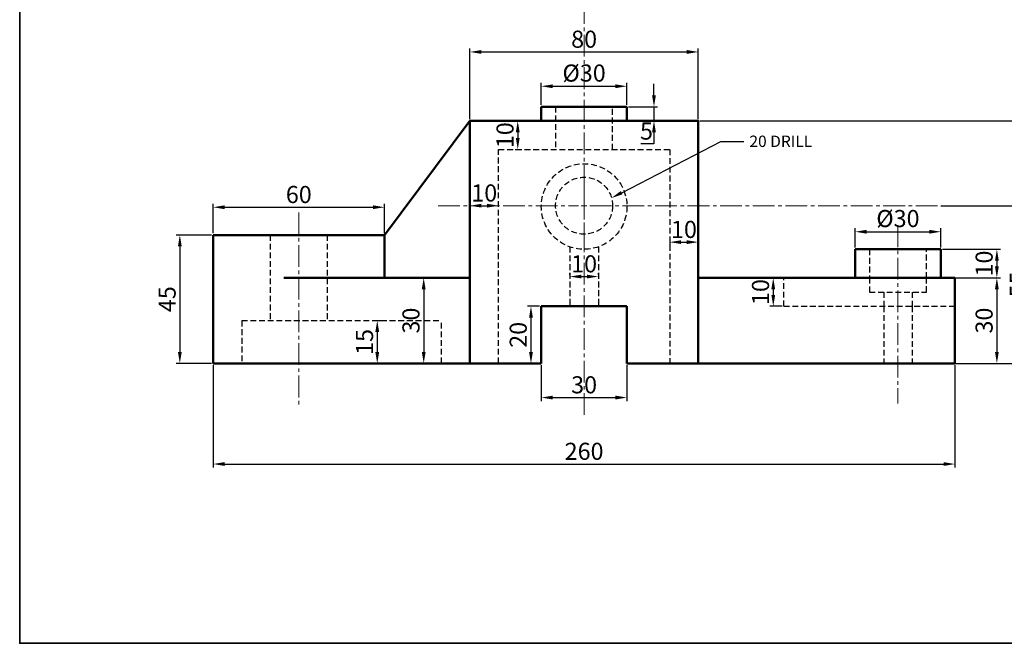
# Model space of a CAD drawing. Units: millimetres. Extents: x 33 to 569, y -180 to 232.
# Tile 1 of 3: x 33 to 378, y -180 to 39. Entities that reach past the tile are written whole.
import ezdxf
from ezdxf import colors
from ezdxf.entities.mleader import LeaderData, LeaderLine
from ezdxf.math import Vec2, Vec3

# ---------------------------------------------------------------- set-up
doc = ezdxf.new("R2010")
doc.units = ezdxf.units.MM
doc.header["$LTSCALE"] = 0.4
doc.linetypes.add('CENTER2', pattern=[28.575, 19.05, -3.175, 3.175, -3.175])
doc.linetypes.add('DASHED', pattern=[19.05, 12.7, -6.35])
for name, color, linetype, lineweight in [('M-CNTR', 1, 'CENTER2', 18), ('M-DIMS', 2, 'Continuous', 25), ('M-HIDN', 4, 'DASHED', 25), ('M-OUTL', 7, 'Continuous', 50), ('M-TEXT', 3, 'Continuous', 25), ('M-TTLB', 7, 'Continuous', 35)]:
    doc.layers.add(name, color=color, linetype=linetype, lineweight=lineweight)
doc.styles.get("Standard").update_dxf_attribs({"font": 'arial.ttf'})
doc.dimstyles.new('ISO-25', dxfattribs={"dimtxt": 6, "dimasz": 4, "dimexe": 1.25, "dimexo": 0.625, "dimtad": 1, "dimtoh": 1, "dimdec": 0, "dimtxsty": 'Standard', "dimcen": 2.5, "dimadec": 0, "dimazin": 0, "dimtfac": 1, "dimtdec": 0, "dimtmove": 0, "dimatfit": 3, "dimfxl": 1, "dimarcsym": 0})

# ---------------------------------------------------------------- blocks, each defined once
blk = doc.blocks.new('*U2')
at = {"layer": 'M-CNTR', "color": 0, "transparency": 16777216}
for p, q in [((0, 2), (0, 92.17)), ((-13.5, 0), (-2, 0)), ((2, 0), (13.5, 0)), ((0, -219.39), (0, -2))]:
    blk.add_line(p, q, dxfattribs=at)
at = {"layer": 'M-CNTR', "color": 0, "linetype": 'Continuous', "transparency": 16777216}
for p, q in [((-1, 0), (1, 0)), ((0, -1), (0, 1))]:
    blk.add_line(p, q, dxfattribs=at)
blk = doc.blocks.new('*U24')
at = {"layer": 'M-CNTR', "color": 0, "transparency": 16777216}
for p, q in [((0, 2), (0, 13.5)), ((-51.2, 0), (-2, 0)), ((2, 0), (124.4, 0)), ((0, -13.5), (0, -2))]:
    blk.add_line(p, q, dxfattribs=at)
at = {"layer": 'M-CNTR', "color": 0, "linetype": 'Continuous', "transparency": 16777216}
for p, q in [((-1, 0), (1, 0)), ((0, -1), (0, 1))]:
    blk.add_line(p, q, dxfattribs=at)
blk = doc.blocks.new('*U25')
at = {"layer": 'M-CNTR', "color": 0, "transparency": 16777216}
blk.add_line((0, 13.4), (0, -49.13), dxfattribs=at)
blk = doc.blocks.new('*U26')
at = {"layer": 'M-CNTR', "color": 0, "transparency": 16777216}
blk.add_line((0, 22.85), (0, -45.4), dxfattribs=at)
blk = doc.blocks.new('*D27')
at = {"layer": 'Defpoints', "color": 0, "ltscale": 0.4, "transparency": 16777216}
for p in [(360.35, -51.65), (360.35, -81.65), (375.03, -81.65)]:
    blk.add_point(p, dxfattribs=at)
at = {"layer": 'M-DIMS', "color": 0, "lineweight": -2, "ltscale": 0.4, "transparency": 16777216}
for p, q in [((360.97, -51.65), (376.28, -51.65)), ((375.03, -55.65), (375.03, -77.65)), ((360.97, -81.65), (376.28, -81.65))]:
    blk.add_line(p, q, dxfattribs=at)
at = {"layer": 'M-DIMS', "color": 0, "ltscale": 0.4, "transparency": 16777216}
for points in [[(374.36, -55.65), (375.69, -55.65), (375.03, -51.65)], [(374.36, -77.65), (375.69, -77.65), (375.03, -81.65)]]:
    blk.add_solid(points, dxfattribs=at)
at = {"layer": 'M-DIMS', "color": 0, "ltscale": 0.4, "transparency": 16777216, "insert": (371.33, -66.65), "char_height": 6, "attachment_point": 5, "rotation": 90}
blk.add_mtext('30', dxfattribs=at)
blk = doc.blocks.new('*D28')
at = {"layer": 'Defpoints', "color": 0, "ltscale": 0.4, "transparency": 16777216}
for p in [(355.35, -41.65), (355.35, -51.65), (375.03, -51.65)]:
    blk.add_point(p, dxfattribs=at)
at = {"layer": 'M-DIMS', "color": 0, "lineweight": -2, "ltscale": 0.4, "transparency": 16777216}
for p, q in [((355.97, -41.65), (376.28, -41.65)), ((375.03, -45.65), (375.03, -47.65)), ((355.97, -51.65), (376.28, -51.65))]:
    blk.add_line(p, q, dxfattribs=at)
at = {"layer": 'M-DIMS', "color": 0, "ltscale": 0.4, "transparency": 16777216}
for points in [[(374.36, -45.65), (375.69, -45.65), (375.03, -41.65)], [(374.36, -47.65), (375.69, -47.65), (375.03, -51.65)]]:
    blk.add_solid(points, dxfattribs=at)
at = {"layer": 'M-DIMS', "color": 0, "ltscale": 0.4, "transparency": 16777216, "insert": (371.34, -46.65), "char_height": 6, "attachment_point": 5, "rotation": 90}
blk.add_mtext('10', dxfattribs=at)
blk = doc.blocks.new('*D29')
at = {"layer": 'Defpoints', "color": 0, "ltscale": 0.4, "transparency": 16777216}
for p in [(354.75, -26.37), (360.35, -81.65), (386.98, -81.65)]:
    blk.add_point(p, dxfattribs=at)
at = {"layer": 'M-DIMS', "color": 0, "lineweight": -2, "ltscale": 0.4, "transparency": 16777216}
for p, q in [((355.37, -26.37), (388.23, -26.37)), ((386.98, -30.37), (386.98, -77.65)), ((360.97, -81.65), (388.23, -81.65))]:
    blk.add_line(p, q, dxfattribs=at)
at = {"layer": 'M-DIMS', "color": 0, "ltscale": 0.4, "transparency": 16777216}
for points in [[(386.31, -30.37), (387.64, -30.37), (386.98, -26.37)], [(386.31, -77.65), (387.64, -77.65), (386.98, -81.65)]]:
    blk.add_solid(points, dxfattribs=at)
at = {"layer": 'M-DIMS', "color": 0, "ltscale": 0.4, "transparency": 16777216, "insert": (383.3, -54.01), "char_height": 6, "attachment_point": 5, "rotation": 90}
blk.add_mtext('55', dxfattribs=at)
blk = doc.blocks.new('*D30')
at = {"layer": 'Defpoints', "color": 0, "ltscale": 0.4, "transparency": 16777216}
for p in [(300.35, -51.65), (296.65, -61.65), (300.35, -61.65)]:
    blk.add_point(p, dxfattribs=at)
at = {"layer": 'M-DIMS', "color": 0, "lineweight": -2, "ltscale": 0.4, "transparency": 16777216}
for p, q in [((299.72, -51.65), (295.4, -51.65)), ((296.65, -55.65), (296.65, -57.65)), ((299.72, -61.65), (295.4, -61.65))]:
    blk.add_line(p, q, dxfattribs=at)
at = {"layer": 'M-DIMS', "color": 0, "ltscale": 0.4, "transparency": 16777216}
for points in [[(295.98, -55.65), (297.32, -55.65), (296.65, -51.65)], [(295.98, -57.65), (297.32, -57.65), (296.65, -61.65)]]:
    blk.add_solid(points, dxfattribs=at)
at = {"layer": 'M-DIMS', "color": 0, "ltscale": 0.4, "transparency": 16777216, "insert": (292.96, -56.65), "char_height": 6, "attachment_point": 5, "rotation": 90}
blk.add_mtext('10', dxfattribs=at)
blk = doc.blocks.new('*D31')
at = {"layer": 'Defpoints', "color": 0, "ltscale": 0.4, "transparency": 16777216}
for p in [(355.35, -35.5), (325.35, -41.65), (355.35, -41.65)]:
    blk.add_point(p, dxfattribs=at)
at = {"layer": 'M-DIMS', "color": 0, "lineweight": -2, "ltscale": 0.4, "transparency": 16777216}
for p, q in [((325.35, -41.02), (325.35, -34.25)), ((355.35, -41.02), (355.35, -34.25)), ((329.35, -35.5), (351.35, -35.5))]:
    blk.add_line(p, q, dxfattribs=at)
at = {"layer": 'M-DIMS', "color": 0, "ltscale": 0.4, "transparency": 16777216}
for points in [[(329.35, -34.83), (329.35, -36.17), (325.35, -35.5)], [(351.35, -34.83), (351.35, -36.17), (355.35, -35.5)]]:
    blk.add_solid(points, dxfattribs=at)
at = {"layer": 'M-DIMS', "color": 0, "ltscale": 0.4, "transparency": 16777216, "insert": (340.35, -31.65), "char_height": 6, "attachment_point": 5}
blk.add_mtext('%%C30', dxfattribs=at)
blk = doc.blocks.new('*D32')
at = {"layer": 'Defpoints', "color": 0, "ltscale": 0.4, "transparency": 16777216}
for p in [(270.35, 3.35), (270.35, -81.65), (398.77, -81.65)]:
    blk.add_point(p, dxfattribs=at)
at = {"layer": 'M-DIMS', "color": 0, "lineweight": -2, "ltscale": 0.4, "transparency": 16777216}
for p, q in [((270.97, 3.35), (400.02, 3.35)), ((398.77, -0.65), (398.77, -77.65)), ((270.97, -81.65), (400.02, -81.65))]:
    blk.add_line(p, q, dxfattribs=at)
at = {"layer": 'M-DIMS', "color": 0, "ltscale": 0.4, "transparency": 16777216}
for points in [[(398.1, -0.65), (399.44, -0.65), (398.77, 3.35)], [(398.1, -77.65), (399.44, -77.65), (398.77, -81.65)]]:
    blk.add_solid(points, dxfattribs=at)
at = {"layer": 'M-DIMS', "color": 0, "ltscale": 0.4, "transparency": 16777216, "insert": (395.08, -39.15), "char_height": 6, "attachment_point": 5, "rotation": 90}
blk.add_mtext('85', dxfattribs=at)
blk = doc.blocks.new('*D33')
at = {"layer": 'Defpoints', "color": 0, "ltscale": 0.4, "transparency": 16777216}
for p in [(245.35, 15.52), (215.35, 8.35), (245.35, 8.35)]:
    blk.add_point(p, dxfattribs=at)
at = {"layer": 'M-DIMS', "color": 0, "lineweight": -2, "ltscale": 0.4, "transparency": 16777216}
for p, q in [((215.35, 8.98), (215.35, 16.77)), ((219.35, 15.52), (241.35, 15.52)), ((245.35, 8.98), (245.35, 16.77))]:
    blk.add_line(p, q, dxfattribs=at)
at = {"layer": 'M-DIMS', "color": 0, "ltscale": 0.4, "transparency": 16777216}
for points in [[(219.35, 16.18), (219.35, 14.85), (215.35, 15.52)], [(241.35, 16.18), (241.35, 14.85), (245.35, 15.52)]]:
    blk.add_solid(points, dxfattribs=at)
at = {"layer": 'M-DIMS', "color": 0, "ltscale": 0.4, "transparency": 16777216, "insert": (230.35, 19.37), "char_height": 6, "attachment_point": 5}
blk.add_mtext('%%C30', dxfattribs=at)
blk = doc.blocks.new('*D34')
at = {"layer": 'Defpoints', "color": 0, "ltscale": 0.4, "transparency": 16777216}
for p in [(270.35, 27.55), (190.35, 3.35), (270.35, 3.35)]:
    blk.add_point(p, dxfattribs=at)
at = {"layer": 'M-DIMS', "color": 0, "lineweight": -2, "ltscale": 0.4, "transparency": 16777216}
for p, q in [((190.35, 3.98), (190.35, 28.8)), ((270.35, 3.98), (270.35, 28.8)), ((194.35, 27.55), (266.35, 27.55))]:
    blk.add_line(p, q, dxfattribs=at)
at = {"layer": 'M-DIMS', "color": 0, "ltscale": 0.4, "transparency": 16777216}
for points in [[(194.35, 28.22), (194.35, 26.88), (190.35, 27.55)], [(266.35, 28.22), (266.35, 26.88), (270.35, 27.55)]]:
    blk.add_solid(points, dxfattribs=at)
at = {"layer": 'M-DIMS', "color": 0, "ltscale": 0.4, "transparency": 16777216, "insert": (230.35, 31.24), "char_height": 6, "attachment_point": 5}
blk.add_mtext('80', dxfattribs=at)
blk = doc.blocks.new('*D35')
at = {"layer": 'Defpoints', "color": 0, "ltscale": 0.4, "transparency": 16777216}
for p in [(245.35, 8.35), (245.35, 3.35), (254.84, 3.35)]:
    blk.add_point(p, dxfattribs=at)
at = {"layer": 'M-DIMS', "color": 0, "lineweight": -2, "ltscale": 0.4, "transparency": 16777216}
for p, q in [((254.84, 12.35), (254.84, 16.35)), ((245.97, 8.35), (256.09, 8.35)), ((254.84, 8.35), (254.84, 3.35)), ((245.97, 3.35), (256.09, 3.35)), ((254.84, -0.65), (254.84, -4.65)), ((254.84, -4.65), (250.24, -4.65))]:
    blk.add_line(p, q, dxfattribs=at)
at = {"layer": 'M-DIMS', "color": 0, "ltscale": 0.4, "transparency": 16777216}
for points in [[(254.17, 12.35), (255.51, 12.35), (254.84, 8.35)], [(254.17, -0.65), (255.51, -0.65), (254.84, 3.35)]]:
    blk.add_solid(points, dxfattribs=at)
at = {"layer": 'M-DIMS', "color": 0, "ltscale": 0.4, "transparency": 16777216, "insert": (252.22, -0.97), "char_height": 6, "attachment_point": 5}
blk.add_mtext('5', dxfattribs=at)
blk = doc.blocks.new('*D36')
at = {"layer": 'Defpoints', "color": 0, "ltscale": 0.4, "transparency": 16777216}
for p in [(205.57, 3.35), (205.57, -6.65), (207.09, -6.65)]:
    blk.add_point(p, dxfattribs=at)
at = {"layer": 'M-DIMS', "color": 0, "lineweight": -2, "ltscale": 0.4, "transparency": 16777216}
for p, q in [((206.19, 3.35), (208.34, 3.35)), ((207.09, -0.65), (207.09, -2.65)), ((206.19, -6.65), (208.34, -6.65))]:
    blk.add_line(p, q, dxfattribs=at)
at = {"layer": 'M-DIMS', "color": 0, "ltscale": 0.4, "transparency": 16777216}
for points in [[(206.43, -0.65), (207.76, -0.65), (207.09, 3.35)], [(206.43, -2.65), (207.76, -2.65), (207.09, -6.65)]]:
    blk.add_solid(points, dxfattribs=at)
at = {"layer": 'M-DIMS', "color": 0, "ltscale": 0.4, "transparency": 16777216, "insert": (203.41, -1.65), "char_height": 6, "attachment_point": 5, "rotation": 90}
blk.add_mtext('10', dxfattribs=at)
blk = doc.blocks.new('*D37')
at = {"layer": 'Defpoints', "color": 0, "ltscale": 0.4, "transparency": 16777216}
for p in [(190.35, -26.37), (200.35, -26.37), (200.35, -26.37)]:
    blk.add_point(p, dxfattribs=at)
at = {"layer": 'M-DIMS', "color": 0, "lineweight": -2, "ltscale": 0.4, "transparency": 16777216}
for p, q in [((190.35, -25.74), (190.35, -25.12)), ((194.35, -26.37), (196.35, -26.37)), ((200.35, -25.74), (200.35, -25.12))]:
    blk.add_line(p, q, dxfattribs=at)
at = {"layer": 'M-DIMS', "color": 0, "ltscale": 0.4, "transparency": 16777216}
for points in [[(194.35, -25.7), (194.35, -27.03), (190.35, -26.37)], [(196.35, -25.7), (196.35, -27.03), (200.35, -26.37)]]:
    blk.add_solid(points, dxfattribs=at)
at = {"layer": 'M-DIMS', "color": 0, "ltscale": 0.4, "transparency": 16777216, "insert": (195.35, -22.68), "char_height": 6, "attachment_point": 5}
blk.add_mtext('10', dxfattribs=at)
blk = doc.blocks.new('*D38')
at = {"layer": 'Defpoints', "color": 0, "ltscale": 0.4, "transparency": 16777216}
for p in [(215.35, -61.65), (211.73, -81.65), (215.35, -81.65)]:
    blk.add_point(p, dxfattribs=at)
at = {"layer": 'M-DIMS', "color": 0, "lineweight": -2, "ltscale": 0.4, "transparency": 16777216}
for p, q in [((214.72, -61.65), (210.48, -61.65)), ((211.73, -65.65), (211.73, -77.65)), ((214.72, -81.65), (210.48, -81.65))]:
    blk.add_line(p, q, dxfattribs=at)
at = {"layer": 'M-DIMS', "color": 0, "ltscale": 0.4, "transparency": 16777216}
for points in [[(211.06, -65.65), (212.4, -65.65), (211.73, -61.65)], [(211.06, -77.65), (212.4, -77.65), (211.73, -81.65)]]:
    blk.add_solid(points, dxfattribs=at)
at = {"layer": 'M-DIMS', "color": 0, "ltscale": 0.4, "transparency": 16777216, "insert": (208.04, -71.65), "char_height": 6, "attachment_point": 5, "rotation": 90}
blk.add_mtext('20', dxfattribs=at)
blk = doc.blocks.new('*D39')
at = {"layer": 'Defpoints', "color": 0, "ltscale": 0.4, "transparency": 16777216}
for p in [(215.35, -81.65), (245.35, -81.65), (245.35, -93.64)]:
    blk.add_point(p, dxfattribs=at)
at = {"layer": 'M-DIMS', "color": 0, "lineweight": -2, "ltscale": 0.4, "transparency": 16777216}
for p, q in [((215.35, -82.27), (215.35, -94.89)), ((245.35, -82.27), (245.35, -94.89)), ((219.35, -93.64), (241.35, -93.64))]:
    blk.add_line(p, q, dxfattribs=at)
at = {"layer": 'M-DIMS', "color": 0, "ltscale": 0.4, "transparency": 16777216}
for points in [[(219.35, -92.98), (219.35, -94.31), (215.35, -93.64)], [(241.35, -92.98), (241.35, -94.31), (245.35, -93.64)]]:
    blk.add_solid(points, dxfattribs=at)
at = {"layer": 'M-DIMS', "color": 0, "ltscale": 0.4, "transparency": 16777216, "insert": (230.35, -89.95), "char_height": 6, "attachment_point": 5}
blk.add_mtext('30', dxfattribs=at)
blk = doc.blocks.new('*D40')
at = {"layer": 'Defpoints', "color": 0, "ltscale": 0.4, "transparency": 16777216}
for p in [(225.35, -51.22), (235.35, -51.22), (235.35, -51.22)]:
    blk.add_point(p, dxfattribs=at)
at = {"layer": 'M-DIMS', "color": 0, "lineweight": -2, "ltscale": 0.4, "transparency": 16777216}
for p, q in [((225.35, -50.59), (225.35, -49.97)), ((229.35, -51.22), (231.35, -51.22)), ((235.35, -50.59), (235.35, -49.97))]:
    blk.add_line(p, q, dxfattribs=at)
at = {"layer": 'M-DIMS', "color": 0, "ltscale": 0.4, "transparency": 16777216}
for points in [[(229.35, -50.55), (229.35, -51.88), (225.35, -51.22)], [(231.35, -50.55), (231.35, -51.88), (235.35, -51.22)]]:
    blk.add_solid(points, dxfattribs=at)
at = {"layer": 'M-DIMS', "color": 0, "ltscale": 0.4, "transparency": 16777216, "insert": (230.35, -47.53), "char_height": 6, "attachment_point": 5}
blk.add_mtext('10', dxfattribs=at)
blk = doc.blocks.new('*D41')
at = {"layer": 'Defpoints', "color": 0, "ltscale": 0.4, "transparency": 16777216}
for p in [(260.35, -38.63), (270.35, -39.15), (270.35, -39.15)]:
    blk.add_point(p, dxfattribs=at)
at = {"layer": 'M-DIMS', "color": 0, "lineweight": -2, "ltscale": 0.4, "transparency": 16777216}
for p, q in [((270.35, -38.52), (270.35, -37.9)), ((260.35, -39.26), (260.35, -40.4)), ((264.35, -39.15), (266.35, -39.15))]:
    blk.add_line(p, q, dxfattribs=at)
at = {"layer": 'M-DIMS', "color": 0, "ltscale": 0.4, "transparency": 16777216}
for points in [[(264.35, -38.48), (264.35, -39.81), (260.35, -39.15)], [(266.35, -38.48), (266.35, -39.81), (270.35, -39.15)]]:
    blk.add_solid(points, dxfattribs=at)
at = {"layer": 'M-DIMS', "color": 0, "ltscale": 0.4, "transparency": 16777216, "insert": (265.35, -35.46), "char_height": 6, "attachment_point": 5}
blk.add_mtext('10', dxfattribs=at)
blk = doc.blocks.new('*D42')
at = {"layer": 'Defpoints', "color": 0, "ltscale": 0.4, "transparency": 16777216}
for p in [(157.39, -66.65), (157.85, -81.65), (157.85, -81.65)]:
    blk.add_point(p, dxfattribs=at)
at = {"layer": 'M-DIMS', "color": 0, "lineweight": -2, "ltscale": 0.4, "transparency": 16777216}
for p, q in [((158.02, -66.65), (159.1, -66.65)), ((157.85, -70.65), (157.85, -77.65)), ((158.47, -81.65), (159.1, -81.65))]:
    blk.add_line(p, q, dxfattribs=at)
at = {"layer": 'M-DIMS', "color": 0, "ltscale": 0.4, "transparency": 16777216}
for points in [[(157.18, -70.65), (158.52, -70.65), (157.85, -66.65)], [(157.18, -77.65), (158.52, -77.65), (157.85, -81.65)]]:
    blk.add_solid(points, dxfattribs=at)
at = {"layer": 'M-DIMS', "color": 0, "ltscale": 0.4, "transparency": 16777216, "insert": (154.16, -74.15), "char_height": 6, "attachment_point": 5, "rotation": 90}
blk.add_mtext('15', dxfattribs=at)
blk = doc.blocks.new('*D43')
at = {"layer": 'Defpoints', "color": 0, "ltscale": 0.4, "transparency": 16777216}
for p in [(171.96, -51.65), (171.96, -81.65), (174.13, -81.65)]:
    blk.add_point(p, dxfattribs=at)
at = {"layer": 'M-DIMS', "color": 0, "lineweight": -2, "ltscale": 0.4, "transparency": 16777216}
for p, q in [((172.58, -51.65), (175.38, -51.65)), ((174.13, -55.65), (174.13, -77.65)), ((172.58, -81.65), (175.38, -81.65))]:
    blk.add_line(p, q, dxfattribs=at)
at = {"layer": 'M-DIMS', "color": 0, "ltscale": 0.4, "transparency": 16777216}
for points in [[(173.47, -55.65), (174.8, -55.65), (174.13, -51.65)], [(173.47, -77.65), (174.8, -77.65), (174.13, -81.65)]]:
    blk.add_solid(points, dxfattribs=at)
at = {"layer": 'M-DIMS', "color": 0, "ltscale": 0.4, "transparency": 16777216, "insert": (170.44, -66.65), "char_height": 6, "attachment_point": 5, "rotation": 90}
blk.add_mtext('30', dxfattribs=at)
blk = doc.blocks.new('*D44')
at = {"layer": 'Defpoints', "color": 0, "ltscale": 0.4, "transparency": 16777216}
for p in [(100.35, -36.65), (88.65, -81.65), (100.35, -81.65)]:
    blk.add_point(p, dxfattribs=at)
at = {"layer": 'M-DIMS', "color": 0, "lineweight": -2, "ltscale": 0.4, "transparency": 16777216}
for p, q in [((99.72, -36.65), (87.4, -36.65)), ((88.65, -40.65), (88.65, -77.65)), ((99.72, -81.65), (87.4, -81.65))]:
    blk.add_line(p, q, dxfattribs=at)
at = {"layer": 'M-DIMS', "color": 0, "ltscale": 0.4, "transparency": 16777216}
for points in [[(87.98, -40.65), (89.32, -40.65), (88.65, -36.65)], [(87.98, -77.65), (89.32, -77.65), (88.65, -81.65)]]:
    blk.add_solid(points, dxfattribs=at)
at = {"layer": 'M-DIMS', "color": 0, "ltscale": 0.4, "transparency": 16777216, "insert": (84.97, -59.15), "char_height": 6, "attachment_point": 5, "rotation": 90}
blk.add_mtext('45', dxfattribs=at)
blk = doc.blocks.new('*D45')
at = {"layer": 'Defpoints', "color": 0, "ltscale": 0.4, "transparency": 16777216}
for p in [(160.35, -26.91), (100.35, -36.65), (160.35, -36.65)]:
    blk.add_point(p, dxfattribs=at)
at = {"layer": 'M-DIMS', "color": 0, "lineweight": -2, "ltscale": 0.4, "transparency": 16777216}
for p, q in [((100.35, -36.02), (100.35, -25.66)), ((104.35, -26.91), (156.35, -26.91)), ((160.35, -36.02), (160.35, -25.66))]:
    blk.add_line(p, q, dxfattribs=at)
at = {"layer": 'M-DIMS', "color": 0, "ltscale": 0.4, "transparency": 16777216}
for points in [[(104.35, -26.24), (104.35, -27.57), (100.35, -26.91)], [(156.35, -26.24), (156.35, -27.57), (160.35, -26.91)]]:
    blk.add_solid(points, dxfattribs=at)
at = {"layer": 'M-DIMS', "color": 0, "ltscale": 0.4, "transparency": 16777216, "insert": (130.35, -23.22), "char_height": 6, "attachment_point": 5}
blk.add_mtext('60', dxfattribs=at)
blk = doc.blocks.new('*D48')
at = {"layer": 'Defpoints', "color": 0, "ltscale": 0.4, "transparency": 16777216}
for p in [(100.35, -81.65), (360.35, -81.65), (360.35, -116.96)]:
    blk.add_point(p, dxfattribs=at)
at = {"layer": 'M-DIMS', "color": 0, "lineweight": -2, "ltscale": 0.4, "transparency": 16777216}
for p, q in [((100.35, -82.27), (100.35, -118.21)), ((360.35, -82.27), (360.35, -118.21)), ((104.35, -116.96), (356.35, -116.96))]:
    blk.add_line(p, q, dxfattribs=at)
at = {"layer": 'M-DIMS', "color": 0, "ltscale": 0.4, "transparency": 16777216}
for points in [[(104.35, -116.29), (104.35, -117.62), (100.35, -116.96)], [(356.35, -116.29), (356.35, -117.62), (360.35, -116.96)]]:
    blk.add_solid(points, dxfattribs=at)
at = {"layer": 'M-DIMS', "color": 0, "ltscale": 0.4, "transparency": 16777216, "insert": (230.35, -113.27), "char_height": 6, "attachment_point": 5}
blk.add_mtext('260', dxfattribs=at)

msp = doc.modelspace()

# ---------------------------------------------------------------- linework, layer by layer
at = {"layer": 'M-HIDN', "ltscale": 0.4}
for p, q in [((220.35, 8.35), (220.35, -6.65)), ((240.35, -6.65), (240.35, 8.35)), ((120.35, -36.65), (120.35, -66.65)), ((140.35, -36.65), (140.35, -66.65)), ((225.35, -40.79), (225.35, -61.65)), ((235.35, -40.79), (235.35, -61.65)), ((300.35, -61.65), (300.35, -51.65)), ((300.35, -61.65), (360.35, -61.65)), ((110.35, -66.65), (110.35, -81.65)), ((110.35, -66.65), (180.35, -66.65)), ((180.35, -81.65), (180.35, -66.65))]:
    msp.add_line(p, q, dxfattribs=at)
for points in [[(200.35, -81.65), (200.35, -6.65), (260.35, -6.65), (260.35, -81.65)], [(330.35, -41.65), (330.35, -51.65), (330.35, -56.65), (350.35, -56.65), (350.35, -51.65), (350.35, -41.65)], [(335.35, -56.65), (335.35, -61.65), (335.35, -81.65)], [(345.35, -56.65), (345.35, -61.65), (345.35, -81.65)]]:
    msp.add_lwpolyline(points, dxfattribs=at)
for centre, radius in [((230.35, -26.65), 15), ((230.35, -26.37), 10)]:
    msp.add_circle(centre, radius, dxfattribs=at)
at = {"layer": 'M-OUTL', "ltscale": 0.4}
for p, q in [((215.35, 8.35), (215.35, 3.35)), ((245.35, 8.35), (215.35, 8.35)), ((245.35, 3.35), (245.35, 8.35)), ((160.35, -36.65), (190.35, 3.35)), ((215.35, 3.35), (245.35, 3.35)), ((100.35, -81.65), (100.35, -36.65)), ((100.35, -36.65), (160.35, -36.65)), ((160.35, -36.65), (160.35, -51.65)), ((325.35, -41.65), (325.35, -51.65)), ((355.35, -41.65), (325.35, -41.65)), ((355.35, -51.65), (355.35, -41.65)), ((160.35, -51.65), (125.12, -51.65)), ((160.35, -51.65), (190.35, -51.65)), ((270.35, -51.65), (360.35, -51.65)), ((360.35, -51.65), (360.35, -81.65)), ((215.35, -81.65), (215.35, -61.65)), ((215.35, -61.65), (245.35, -61.65)), ((245.35, -61.65), (245.35, -81.65)), ((100.35, -81.65), (215.35, -81.65)), ((245.35, -81.65), (360.35, -81.65))]:
    msp.add_line(p, q, dxfattribs=at)
msp.add_lwpolyline([(190.35, -81.65), (190.35, 3.35), (270.35, 3.35), (270.35, -81.65)], dxfattribs=at)
at = {"layer": 'M-TTLB', "ltscale": 0.4}
msp.add_lwpolyline([(568.64, -179.82), (32.52, -179.82), (32.52, 232.48), (568.64, 232.48)], close=True, dxfattribs=at)

# ---------------------------------------------------------------- block references
at = {"layer": 'M-CNTR'}
for name, p in [('*U2', (230.35, 119.63)), ('*U24', (230.35, -26.37)), ('*U26', (130.35, -51.65)), ('*U25', (340.35, -46.65))]:
    msp.add_blockref(name, p, dxfattribs=at)

# ---------------------------------------------------------------- dimensions: what is measured, and where the dimension line sits
at = {"layer": 'M-DIMS', "ltscale": 0.4}
for base, p1, p2, override, picture, middle in [((270.35, 27.55), (190.35, 3.35), (270.35, 3.35), {"dimclrd": 0, "dimclre": 0, "dimclrt": 0}, '*D34', (230.35, 31.24)), ((160.35, -26.91), (100.35, -36.65), (160.35, -36.65), {"dimclrd": 0, "dimclre": 0, "dimclrt": 0}, '*D45', (130.35, -23.22)), ((200.35, -26.37), (190.35, -26.37), (200.35, -26.37), {"dimclrd": 0, "dimclre": 0, "dimclrt": 0}, '*D37', (195.35, -22.68)), ((270.35, -39.15), (260.35, -38.63), (270.35, -39.15), {"dimclrd": 0, "dimclre": 0, "dimclrt": 0}, '*D41', (265.35, -35.46)), ((235.35, -51.22), (225.35, -51.22), (235.35, -51.22), {"dimclrd": 0, "dimclre": 0, "dimclrt": 0}, '*D40', (230.35, -47.53)), ((360.35, -116.96), (100.35, -81.65), (360.35, -81.65), {"dimdec": 0, "dimlfac": 1, "dimrnd": 0, "dimzin": 0, "dimdsep": 46, "dimlunit": 2}, '*D48', (230.35, -113.27)), ((245.35, -93.64), (215.35, -81.65), (245.35, -81.65), {"dimclrd": 0, "dimclre": 0, "dimclrt": 0}, '*D39', (230.35, -89.95))]:
    dim = msp.add_linear_dim(base=base, p1=p1, p2=p2, dimstyle='ISO-25', override=override, dxfattribs=at)
    dim.commit()
    dim.dimension.update_dxf_attribs({"geometry": picture, "text_midpoint": middle})
for base, p1, p2, picture, middle in [((245.35, 15.52), (215.35, 8.35), (245.35, 8.35), '*D33', (230.35, 19.37)), ((355.35, -35.5), (325.35, -41.65), (355.35, -41.65), '*D31', (340.35, -31.65))]:
    dim = msp.add_linear_dim(base=base, p1=p1, p2=p2, text='%%C<>', dimstyle='ISO-25', override={"dimclrd": 0, "dimclre": 0, "dimclrt": 0}, dxfattribs=at)
    dim.commit()
    dim.dimension.update_dxf_attribs({"geometry": picture, "text_midpoint": middle})
for base, p1, p2, picture, middle in [((254.84, 3.35), (245.35, 8.35), (245.35, 3.35), '*D35', (252.22, -0.97)), ((207.09, -6.65), (205.57, 3.35), (205.57, -6.65), '*D36', (203.41, -1.65)), ((398.77, -81.65), (270.35, 3.35), (270.35, -81.65), '*D32', (395.08, -39.15)), ((386.98, -81.65), (354.75, -26.37), (360.35, -81.65), '*D29', (383.3, -54.01)), ((88.65, -81.65), (100.35, -36.65), (100.35, -81.65), '*D44', (84.97, -59.15)), ((375.03, -51.65), (355.35, -41.65), (355.35, -51.65), '*D28', (371.34, -46.65)), ((174.13, -81.65), (171.96, -51.65), (171.96, -81.65), '*D43', (170.44, -66.65)), ((296.65, -61.65), (300.35, -51.65), (300.35, -61.65), '*D30', (292.96, -56.65)), ((375.03, -81.65), (360.35, -51.65), (360.35, -81.65), '*D27', (371.33, -66.65)), ((211.73, -81.65), (215.35, -61.65), (215.35, -81.65), '*D38', (208.04, -71.65)), ((157.85, -81.65), (157.39, -66.65), (157.85, -81.65), '*D42', (154.16, -74.15))]:
    dim = msp.add_linear_dim(base=base, p1=p1, p2=p2, angle=90, dimstyle='ISO-25', override={"dimclrd": 0, "dimclre": 0, "dimclrt": 0}, dxfattribs=at)
    dim.commit()
    dim.dimension.update_dxf_attribs({"geometry": picture, "text_midpoint": middle})

# ---------------------------------------------------------------- leaders
at = {"layer": 'M-TEXT', "ltscale": 0.4}
ml = msp.add_multileader_mtext('Standard', dxfattribs=at)
ml.set_content('20 DRILL', color=256)
ml.set_leader_properties()
ml.build(insert=Vec2(0, 0))
ctx = ml.context
ctx.base_point, ctx.plane_origin = Vec3(286.29, -3.83), Vec3(239.97, -23.64)
notes = []
notes.append((ctx, [(0, (1, 1, 0), (278.29, -3.83), (1, 0), 8, [(0, [(239.97, -23.64)], 0, [])])]))
ctx.mtext.insert, ctx.mtext.flow_direction = Vec3(288.29, -1.79), 5
for ctx, leaders in notes:
    for number, flags, end, landing, length, lines in leaders:
        leader = LeaderData()
        leader.index, (leader.has_last_leader_line, leader.has_dogleg_vector, leader.attachment_direction) = number, flags
        leader.last_leader_point, leader.dogleg_vector, leader.dogleg_length = Vec3(end), Vec3(landing), length
        for number, points, colour, breaks in lines:
            line = LeaderLine()
            line.index, line.vertices, line.color, line.breaks = number, Vec3.list(points), colors.encode_raw_color(colour), breaks
            leader.lines.append(line)
        ctx.leaders.append(leader)

doc.saveas('drawing.dxf')
